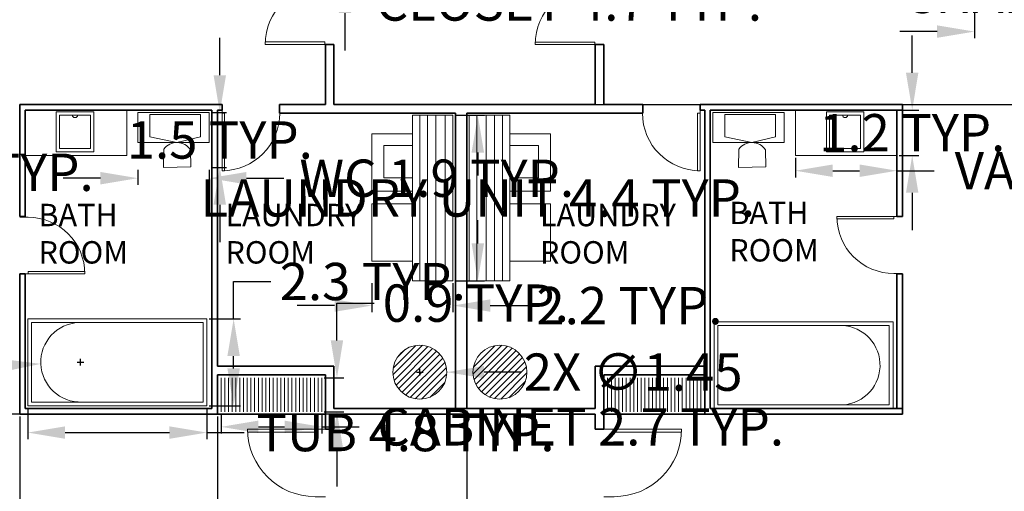
# Model space of a CAD drawing. Units: metres. Extents: x 25.1 to 96.1, y 24.3 to 71.3.
# Tile 3 of 5: x 45.8 to 72.2, y 43.8 to 56.5. Entities that reach past the tile are written whole.
import ezdxf

# ---------------------------------------------------------------- set-up
doc = ezdxf.new("R2010")
doc.units = ezdxf.units.M
doc.header["$MEASUREMENT"] = 0
for name, color, linetype, lineweight in [('A-AREA-IDEN', 1, 'Continuous', 18), ('A-EQPM', 163, 'Continuous', 18), ('A-EQPM-PATT', 152, 'Continuous', 13), ('A-FLOR-CASE', 8, 'Continuous', 18), ('A-FLOR-FIXT', 163, 'Continuous', 18), ('A-WALL', 7, 'Continuous', 35), ('dimension', 80, 'Continuous', 18), ('door', 17, 'Continuous', 18), ('furniture', 163, 'Continuous', 18)]:
    doc.layers.add(name, color=color, linetype=linetype, lineweight=lineweight)
doc.styles.get("Standard").update_dxf_attribs({"font": 'arial.ttf'})
doc.dimstyles.get("Standard").update_dxf_attribs({"dimtxt": 1, "dimasz": 1, "dimexe": 0.18, "dimexo": 0.0625, "dimgap": 0.09, "dimtad": 0, "dimtih": 1, "dimtoh": 1, "dimdec": 1, "dimzin": 0, "dimdsep": 46, "dimtxsty": 'Standard', "dimcen": 0.09, "dimadec": 0, "dimazin": 0, "dimtfac": 1, "dimtdec": 1, "dimtofl": 0, "dimtmove": 0, "dimatfit": 3, "dimfxl": 1, "dimtolj": 1, "dimtzin": 0, "dimarcsym": 0})

# ---------------------------------------------------------------- blocks, each defined once
blk = doc.blocks.new('t')
for points in [[(29.887, -1.464), (34.681, -1.464), (34.681, 0.864), (29.887, 0.864)], [(29.987, -1.364), (34.581, -1.364), (34.581, 0.764), (29.987, 0.764)]]:
    blk.add_lwpolyline(points, close=True)
blk.add_arc((31.299, -0.3), 1.065, 92.3033, 272.3033)
blk = doc.blocks.new('fff')
at = {"layer": 'furniture'}
for p, q in [((35.063, -0.715), (35.063, -1.625)), ((35.163, -0.715), (35.163, -1.625)), ((35.263, -0.715), (35.263, -1.625)), ((35.363, -0.715), (35.363, -1.625)), ((35.463, -0.715), (35.463, -1.625)), ((35.563, -0.715), (35.563, -1.625)), ((35.663, -0.715), (35.663, -1.625)), ((35.763, -0.715), (35.763, -1.625)), ((35.863, -0.715), (35.863, -1.625)), ((35.963, -0.715), (35.963, -1.625)), ((36.063, -0.715), (36.063, -1.625)), ((36.163, -0.715), (36.163, -1.625)), ((36.263, -0.715), (36.263, -1.625)), ((36.363, -0.715), (36.363, -1.625)), ((36.463, -0.715), (36.463, -1.625)), ((36.563, -0.715), (36.563, -1.625)), ((36.663, -0.715), (36.663, -1.625)), ((36.763, -0.715), (36.763, -1.625)), ((36.863, -0.715), (36.863, -1.625)), ((36.963, -0.715), (36.963, -1.625)), ((37.063, -0.715), (37.063, -1.625)), ((37.163, -0.715), (37.163, -1.625)), ((37.263, -0.715), (37.263, -1.625)), ((37.363, -0.715), (37.363, -1.625)), ((37.463, -0.715), (37.463, -1.625)), ((37.563, -0.715), (37.563, -1.625)), ((37.663, -0.715), (37.663, -1.625)), ((37.763, -0.715), (37.763, -1.625))]:
    blk.add_line(p, q, dxfattribs=at)
blk = doc.blocks.new('sinn')
for points in [[(29.82, 6.458), (32.54, 6.458), (32.54, 5.24), (29.82, 5.24)], [(30.649, 6.409), (31.653, 6.409), (31.653, 5.34), (30.649, 5.34)], [(30.734, 6.324), (31.567, 6.324), (31.567, 5.426), (30.734, 5.426)]]:
    blk.add_lwpolyline(points, close=True)
blk.add_arc((31.151, 6.324), 0.0703, 180, 0)
blk = doc.blocks.new('wc')
for p, q in [((33.157, 5.739), (33.883, 5.588)), ((33.883, 5.588), (34.514, 5.739)), ((33.535, 5.411), (33.522, 4.918)), ((34.255, 4.935), (34.244, 5.394)), ((33.522, 4.918), (34.255, 4.935))]:
    blk.add_line(p, q)
blk.add_lwpolyline([(32.833, 6.392), (34.743, 6.392), (34.743, 5.588), (32.833, 5.588)], close=True)
blk.add_lwpolyline([(33.157, 5.739), (33.157, 6.335), (34.514, 6.335), (34.514, 5.739)])
blk.add_arc((33.883, 5.156), 0.432, 33.4958, 143.723)
blk = doc.blocks.new('w')
at = {"layer": 'furniture'}
for p, q in [((40.384, 1.885), (40.384, 6.319)), ((40.596, 1.885), (40.596, 6.319)), ((40.82, 1.885), (40.82, 6.319)), ((40.82, 1.885), (40.82, 6.319)), ((41.069, 1.885), (41.069, 6.319))]:
    blk.add_line(p, q, dxfattribs=at)
for points in [[(41.275, 6.319), (40.188, 6.319), (40.188, 1.885), (41.275, 1.885)], [(40.188, 5.819), (39.103, 5.819), (39.103, 4.287), (40.188, 4.287)], [(40.188, 5.51), (39.421, 5.51), (39.421, 4.637), (40.188, 4.637)], [(40.188, 3.945), (39.103, 3.945), (39.103, 2.413), (40.188, 2.413)]]:
    blk.add_lwpolyline(points, close=True, dxfattribs=at)
blk = doc.blocks.new('*U22')
for p, q in [((0, 0), (0, -6)), ((40, 0), (40, -6))]:
    blk.add_line(p, q)
blk.add_lwpolyline([(0, 0), (0, 40), (1.75, 40), (1.75, 0)], close=True)
blk.add_arc((0, 0), 40, 0, 90)
blk = doc.blocks.new('*D34')
at = {"layer": 'Defpoints', "color": 0, "transparency": 16777216}
for p in [(46.002, 46.126), (50.795, 46.126), (50.795, 45.407)]:
    blk.add_point(p, dxfattribs=at)
at = {"layer": 'dimension', "color": 0, "lineweight": -2, "transparency": 16777216}
for p, q in [((46.002, 46.063), (46.002, 45.227)), ((50.795, 46.063), (50.795, 45.227)), ((47.002, 45.407), (49.795, 45.407)), ((50.795, 45.407), (51.795, 45.407))]:
    blk.add_line(p, q, dxfattribs=at)
at = {"layer": 'dimension', "color": 0, "transparency": 16777216}
for points in [[(47.002, 45.573), (47.002, 45.24), (46.002, 45.407)], [(49.795, 45.573), (49.795, 45.24), (50.795, 45.407)]]:
    blk.add_solid(points, dxfattribs=at)
at = {"layer": 'dimension', "color": 0, "transparency": 16777216, "insert": (56.117, 45.407), "char_height": 1, "attachment_point": 5}
blk.add_mtext('\\A1;TUB 4.8 TYP.', dxfattribs=at)
blk = doc.blocks.new('*D35')
at = {"layer": 'Defpoints', "color": 0, "transparency": 16777216}
for p in [(50.795, 48.454), (51.514, 48.454), (50.795, 46.126)]:
    blk.add_point(p, dxfattribs=at)
at = {"layer": 'dimension', "color": 0, "lineweight": -2, "transparency": 16777216}
for p, q in [((51.514, 48.454), (51.514, 49.454)), ((51.514, 49.454), (52.514, 49.454)), ((50.858, 48.454), (51.694, 48.454)), ((51.514, 47.126), (51.514, 47.454)), ((50.858, 46.126), (51.694, 46.126))]:
    blk.add_line(p, q, dxfattribs=at)
at = {"layer": 'dimension', "color": 0, "transparency": 16777216}
for points in [[(51.347, 47.454), (51.681, 47.454), (51.514, 48.454)], [(51.347, 47.126), (51.681, 47.126), (51.514, 46.126)]]:
    blk.add_solid(points, dxfattribs=at)
at = {"layer": 'dimension', "color": 0, "transparency": 16777216, "insert": (55.24, 49.454), "char_height": 1, "attachment_point": 5}
blk.add_mtext('\\A1;2.3 TYP.', dxfattribs=at)
blk = doc.blocks.new('*D37')
at = {"layer": 'Defpoints', "color": 0, "transparency": 16777216}
for p in [(71.357, 57.619), (72.431, 57.619), (72.431, 56.149)]:
    blk.add_point(p, dxfattribs=at)
at = {"layer": 'dimension', "color": 0, "lineweight": -2, "transparency": 16777216}
for p, q in [((71.357, 57.557), (71.357, 55.969)), ((72.431, 57.557), (72.431, 55.969)), ((70.357, 56.149), (69.357, 56.149)), ((73.431, 56.149), (74.431, 56.149))]:
    blk.add_line(p, q, dxfattribs=at)
at = {"layer": 'dimension', "color": 0, "transparency": 16777216}
for points in [[(70.357, 56.316), (70.357, 55.982), (71.357, 56.149)], [(73.431, 56.316), (73.431, 55.982), (72.431, 56.149)]]:
    blk.add_solid(points, dxfattribs=at)
at = {"layer": 'dimension', "color": 0, "transparency": 16777216, "insert": (77.102, 56.149), "char_height": 1, "attachment_point": 5}
blk.add_mtext('\\A1;1.1 TYP.', dxfattribs=at)
blk = doc.blocks.new('*D44')
at = {"layer": 'Defpoints', "color": 0, "transparency": 16777216}
for p in [(35.843, 52.744), (38.271, 52.744), (38.271, 52.38)]:
    blk.add_point(p, dxfattribs=at)
at = {"layer": 'dimension', "color": 0, "lineweight": -2, "transparency": 16777216}
for p, q in [((35.843, 52.682), (35.843, 52.2)), ((38.271, 52.682), (38.271, 52.2)), ((36.843, 52.38), (37.271, 52.38)), ((38.271, 52.38), (39.271, 52.38))]:
    blk.add_line(p, q, dxfattribs=at)
at = {"layer": 'dimension', "color": 0, "transparency": 16777216}
for points in [[(36.843, 52.547), (36.843, 52.213), (35.843, 52.38)], [(37.271, 52.547), (37.271, 52.213), (38.271, 52.38)]]:
    blk.add_solid(points, dxfattribs=at)
at = {"layer": 'dimension', "color": 0, "transparency": 16777216, "insert": (43.67, 52.38), "char_height": 1, "attachment_point": 5}
blk.add_mtext('\\A1;HOB 2.4 TYP.', dxfattribs=at)
blk = doc.blocks.new('*D48')
at = {"layer": 'Defpoints', "color": 0, "transparency": 16777216}
for p in [(80.148, 57.146), (80.148, 56.81), (82.383, 56.81)]:
    blk.add_point(p, dxfattribs=at)
at = {"layer": 'dimension', "color": 0, "lineweight": -2, "transparency": 16777216}
for p, q in [((80.148, 56.873), (80.148, 57.326)), ((82.383, 56.873), (82.383, 57.326)), ((80.148, 57.146), (79.148, 57.146)), ((81.383, 57.146), (81.148, 57.146))]:
    blk.add_line(p, q, dxfattribs=at)
at = {"layer": 'dimension', "color": 0, "transparency": 16777216}
for points in [[(81.148, 57.312), (81.148, 56.979), (80.148, 57.146)], [(81.383, 57.312), (81.383, 56.979), (82.383, 57.146)]]:
    blk.add_solid(points, dxfattribs=at)
at = {"layer": 'dimension', "color": 0, "transparency": 16777216, "insert": (74.068, 57.146), "char_height": 1, "attachment_point": 5}
blk.add_mtext('\\A1;CHAIR 2.2 TYP.', dxfattribs=at)
blk = doc.blocks.new('*D56')
at = {"layer": 'Defpoints', "color": 0, "transparency": 16777216}
for p in [(49.092, 57.646), (53.792, 57.646), (53.792, 56.941)]:
    blk.add_point(p, dxfattribs=at)
at = {"layer": 'dimension', "color": 0, "lineweight": -2, "transparency": 16777216}
for p, q in [((49.092, 57.584), (49.092, 56.761)), ((53.792, 57.584), (53.792, 56.761)), ((50.092, 56.941), (52.792, 56.941)), ((53.792, 56.941), (54.792, 56.941))]:
    blk.add_line(p, q, dxfattribs=at)
at = {"layer": 'dimension', "color": 0, "transparency": 16777216}
for points in [[(50.092, 57.108), (50.092, 56.774), (49.092, 56.941)], [(52.792, 57.108), (52.792, 56.774), (53.792, 56.941)]]:
    blk.add_solid(points, dxfattribs=at)
at = {"layer": 'dimension', "color": 0, "transparency": 16777216, "insert": (60.493, 56.941), "char_height": 1, "attachment_point": 5}
blk.add_mtext('\\A1;CLOSET 4.7 TYP.', dxfattribs=at)
blk = doc.blocks.new('*D57')
at = {"layer": 'Defpoints', "color": 0, "transparency": 16777216}
for p in [(53.792, 58.716), (54.497, 58.716), (53.792, 57.646)]:
    blk.add_point(p, dxfattribs=at)
at = {"layer": 'dimension', "color": 0, "lineweight": -2, "transparency": 16777216}
for p, q in [((54.497, 59.716), (54.497, 60.716)), ((54.497, 60.716), (55.497, 60.716)), ((53.855, 58.716), (54.677, 58.716)), ((53.855, 57.646), (54.677, 57.646)), ((54.497, 56.646), (54.497, 55.646))]:
    blk.add_line(p, q, dxfattribs=at)
at = {"layer": 'dimension', "color": 0, "transparency": 16777216}
for points in [[(54.331, 59.716), (54.664, 59.716), (54.497, 58.716)], [(54.331, 56.646), (54.664, 56.646), (54.497, 57.646)]]:
    blk.add_solid(points, dxfattribs=at)
at = {"layer": 'dimension', "color": 0, "transparency": 16777216, "insert": (58.168, 60.716), "char_height": 1, "attachment_point": 5}
blk.add_mtext('\\A1;1.1 TYP.', dxfattribs=at)
blk = doc.blocks.new('*D58')
at = {"layer": 'Defpoints', "color": 0, "transparency": 16777216}
for p in [(51.177, 45.965), (53.877, 45.965), (53.877, 45.56)]:
    blk.add_point(p, dxfattribs=at)
at = {"layer": 'dimension', "color": 0, "lineweight": -2, "transparency": 16777216}
for p, q in [((51.177, 45.903), (51.177, 45.38)), ((53.877, 45.903), (53.877, 45.38)), ((52.177, 45.56), (52.877, 45.56)), ((53.877, 45.56), (54.877, 45.56))]:
    blk.add_line(p, q, dxfattribs=at)
at = {"layer": 'dimension', "color": 0, "transparency": 16777216}
for points in [[(52.177, 45.727), (52.177, 45.394), (51.177, 45.56)], [(52.877, 45.727), (52.877, 45.394), (53.877, 45.56)]]:
    blk.add_solid(points, dxfattribs=at)
at = {"layer": 'dimension', "color": 0, "transparency": 16777216, "insert": (60.81, 45.56), "char_height": 1, "attachment_point": 5}
blk.add_mtext('\\A1;CABINET 2.7 TYP.', dxfattribs=at)
blk = doc.blocks.new('*D59')
at = {"layer": 'Defpoints', "color": 0, "transparency": 16777216}
for p in [(53.877, 46.875), (54.282, 46.875), (53.877, 45.965)]:
    blk.add_point(p, dxfattribs=at)
at = {"layer": 'dimension', "color": 0, "lineweight": -2, "transparency": 16777216}
for p, q in [((54.282, 47.875), (54.282, 48.875)), ((54.282, 48.875), (55.282, 48.875)), ((53.939, 46.875), (54.462, 46.875)), ((53.939, 45.965), (54.462, 45.965)), ((54.282, 44.965), (54.282, 43.965))]:
    blk.add_line(p, q, dxfattribs=at)
at = {"layer": 'dimension', "color": 0, "transparency": 16777216}
for points in [[(54.115, 47.875), (54.448, 47.875), (54.282, 46.875)], [(54.115, 44.965), (54.448, 44.965), (54.282, 45.965)]]:
    blk.add_solid(points, dxfattribs=at)
at = {"layer": 'dimension', "color": 0, "transparency": 16777216, "insert": (58, 48.875), "char_height": 1, "attachment_point": 5}
blk.add_mtext('\\A1;0.9 TYP.', dxfattribs=at)
blk = doc.blocks.new('*D60')
at = {"layer": 'Defpoints', "color": 0, "transparency": 16777216}
for p in [(66.561, 52.83), (69.281, 52.83), (69.281, 52.422)]:
    blk.add_point(p, dxfattribs=at)
at = {"layer": 'dimension', "color": 0, "lineweight": -2, "transparency": 16777216}
for p, q in [((66.561, 52.767), (66.561, 52.242)), ((69.281, 52.767), (69.281, 52.242)), ((67.561, 52.422), (68.281, 52.422)), ((69.281, 52.422), (70.281, 52.422))]:
    blk.add_line(p, q, dxfattribs=at)
at = {"layer": 'dimension', "color": 0, "transparency": 16777216}
for points in [[(67.561, 52.588), (67.561, 52.255), (66.561, 52.422)], [(68.281, 52.588), (68.281, 52.255), (69.281, 52.422)]]:
    blk.add_solid(points, dxfattribs=at)
at = {"layer": 'dimension', "color": 0, "transparency": 16777216, "insert": (75.742, 52.422), "char_height": 1, "attachment_point": 5}
blk.add_mtext('\\A1;VANITY 2.7 TYP.', dxfattribs=at)
blk = doc.blocks.new('*D61')
at = {"layer": 'Defpoints', "color": 0, "transparency": 16777216}
for p in [(69.281, 54.048), (69.689, 54.048), (69.281, 52.83)]:
    blk.add_point(p, dxfattribs=at)
at = {"layer": 'dimension', "color": 0, "lineweight": -2, "transparency": 16777216}
for p, q in [((69.689, 55.048), (69.689, 56.048)), ((69.343, 54.048), (69.869, 54.048)), ((69.343, 52.83), (69.869, 52.83)), ((69.689, 51.83), (69.689, 50.83))]:
    blk.add_line(p, q, dxfattribs=at)
at = {"layer": 'dimension', "color": 0, "transparency": 16777216}
for points in [[(69.522, 55.048), (69.855, 55.048), (69.689, 54.048)], [(69.522, 51.83), (69.855, 51.83), (69.689, 52.83)]]:
    blk.add_solid(points, dxfattribs=at)
at = {"layer": 'dimension', "color": 0, "transparency": 16777216, "insert": (69.689, 53.439), "char_height": 1, "attachment_point": 5}
blk.add_mtext('\\A1;1.2 TYP.', dxfattribs=at)
blk = doc.blocks.new('*D62')
at = {"layer": 'Defpoints', "color": 0, "transparency": 16777216}
for p in [(48.947, 52.508), (50.857, 52.508), (50.857, 52.221)]:
    blk.add_point(p, dxfattribs=at)
at = {"layer": 'dimension', "color": 0, "lineweight": -2, "transparency": 16777216}
for p, q in [((47.947, 52.221), (46.947, 52.221)), ((48.947, 52.446), (48.947, 52.041)), ((50.857, 52.446), (50.857, 52.041)), ((51.857, 52.221), (52.857, 52.221))]:
    blk.add_line(p, q, dxfattribs=at)
at = {"layer": 'dimension', "color": 0, "transparency": 16777216}
for points in [[(47.947, 52.388), (47.947, 52.055), (48.947, 52.221)], [(51.857, 52.388), (51.857, 52.055), (50.857, 52.221)]]:
    blk.add_solid(points, dxfattribs=at)
at = {"layer": 'dimension', "color": 0, "transparency": 16777216, "insert": (56.954, 52.221), "char_height": 1, "attachment_point": 5}
blk.add_mtext('\\A1;WC 1.9 TYP.', dxfattribs=at)
blk = doc.blocks.new('*D63')
at = {"layer": 'Defpoints', "color": 0, "transparency": 16777216}
for p in [(50.857, 53.981), (51.144, 53.981), (50.857, 52.508)]:
    blk.add_point(p, dxfattribs=at)
at = {"layer": 'dimension', "color": 0, "lineweight": -2, "transparency": 16777216}
for p, q in [((51.144, 54.981), (51.144, 55.981)), ((50.92, 53.981), (51.324, 53.981)), ((50.92, 52.508), (51.324, 52.508)), ((51.144, 51.508), (51.144, 50.508))]:
    blk.add_line(p, q, dxfattribs=at)
at = {"layer": 'dimension', "color": 0, "transparency": 16777216}
for points in [[(50.977, 54.981), (51.311, 54.981), (51.144, 53.981)], [(50.977, 51.508), (51.311, 51.508), (51.144, 52.508)]]:
    blk.add_solid(points, dxfattribs=at)
at = {"layer": 'dimension', "color": 0, "transparency": 16777216, "insert": (51.144, 53.245), "char_height": 1, "attachment_point": 5}
blk.add_mtext('\\A1;1.5 TYP.', dxfattribs=at)
blk = doc.blocks.new('*D64')
at = {"layer": 'Defpoints', "color": 0, "transparency": 16777216}
for p in [(57.389, 53.909), (58.055, 53.909), (57.389, 49.475)]:
    blk.add_point(p, dxfattribs=at)
at = {"layer": 'dimension', "color": 0, "lineweight": -2, "transparency": 16777216}
for p, q in [((57.452, 53.909), (58.235, 53.909)), ((58.055, 52.909), (58.055, 52.29)), ((58.055, 50.475), (58.055, 51.093)), ((57.452, 49.475), (58.235, 49.475))]:
    blk.add_line(p, q, dxfattribs=at)
at = {"layer": 'dimension', "color": 0, "transparency": 16777216}
for points in [[(57.888, 52.909), (58.221, 52.909), (58.055, 53.909)], [(57.888, 50.475), (58.221, 50.475), (58.055, 49.475)]]:
    blk.add_solid(points, dxfattribs=at)
at = {"layer": 'dimension', "color": 0, "transparency": 16777216, "insert": (58.055, 51.692), "char_height": 1, "attachment_point": 5}
blk.add_mtext('\\A1;LAUNDRY UNIT 4.4 TYP.', dxfattribs=at)
blk = doc.blocks.new('*D65')
at = {"layer": 'Defpoints', "color": 0, "transparency": 16777216}
for p in [(55.217, 49.475), (57.389, 49.475), (57.389, 48.809)]:
    blk.add_point(p, dxfattribs=at)
at = {"layer": 'dimension', "color": 0, "lineweight": -2, "transparency": 16777216}
for p, q in [((55.217, 49.412), (55.217, 48.629)), ((57.389, 49.412), (57.389, 48.629)), ((54.217, 48.809), (53.217, 48.809)), ((58.389, 48.809), (59.389, 48.809))]:
    blk.add_line(p, q, dxfattribs=at)
at = {"layer": 'dimension', "color": 0, "transparency": 16777216}
for points in [[(54.217, 48.976), (54.217, 48.643), (55.217, 48.809)], [(58.389, 48.976), (58.389, 48.643), (57.389, 48.809)]]:
    blk.add_solid(points, dxfattribs=at)
at = {"layer": 'dimension', "color": 0, "transparency": 16777216, "insert": (62.116, 48.809), "char_height": 1, "attachment_point": 5}
blk.add_mtext('\\A1;2.2 TYP.', dxfattribs=at)
blk = doc.blocks.new('*D78')
at = {"layer": 'Defpoints', "color": 0, "transparency": 16777216}
for p in [(45.784, 45.898), (51.084, 45.898), (51.084, 24.973)]:
    blk.add_point(p, dxfattribs=at)
at = {"layer": 'dimension', "color": 0, "lineweight": -2, "transparency": 16777216}
for p, q in [((45.784, 45.835), (45.784, 24.793)), ((51.084, 45.835), (51.084, 24.793)), ((46.784, 24.973), (47.434, 24.973)), ((50.084, 24.973), (49.434, 24.973))]:
    blk.add_line(p, q, dxfattribs=at)
at = {"layer": 'dimension', "color": 0, "transparency": 16777216}
for points in [[(46.784, 25.139), (46.784, 24.806), (45.784, 24.973)], [(50.084, 25.139), (50.084, 24.806), (51.084, 24.973)]]:
    blk.add_solid(points, dxfattribs=at)
at = {"layer": 'dimension', "color": 0, "transparency": 16777216, "insert": (48.434, 24.973), "char_height": 1, "attachment_point": 5}
blk.add_mtext('\\A1;5.3', dxfattribs=at)
blk = doc.blocks.new('*D79')
at = {"layer": 'Defpoints', "color": 0, "transparency": 16777216}
for p in [(51.084, 45.898), (57.757, 46.048), (57.757, 24.973)]:
    blk.add_point(p, dxfattribs=at)
at = {"layer": 'dimension', "color": 0, "lineweight": -2, "transparency": 16777216}
for p, q in [((57.757, 45.985), (57.757, 24.793)), ((51.084, 45.835), (51.084, 24.793)), ((52.084, 24.973), (52.641, 24.973)), ((56.757, 24.973), (56.201, 24.973))]:
    blk.add_line(p, q, dxfattribs=at)
at = {"layer": 'dimension', "color": 0, "transparency": 16777216}
for points in [[(52.084, 25.139), (52.084, 24.806), (51.084, 24.973)], [(56.757, 25.139), (56.757, 24.806), (57.757, 24.973)]]:
    blk.add_solid(points, dxfattribs=at)
at = {"layer": 'dimension', "color": 0, "transparency": 16777216, "insert": (54.421, 24.973), "char_height": 1, "attachment_point": 5}
blk.add_mtext('\\A1;6.673', dxfattribs=at)
blk = doc.blocks.new('*D84')
at = {"layer": 'Defpoints', "color": 0, "transparency": 16777216}
for p in [(29.225, 45.898), (61.201, 45.898), (61.201, 32.464)]:
    blk.add_point(p, dxfattribs=at)
at = {"layer": 'dimension', "color": 0, "lineweight": -2, "transparency": 16777216}
for p, q in [((61.138, 45.898), (29.045, 45.898)), ((29.225, 44.898), (29.225, 39.781)), ((29.225, 33.464), (29.225, 38.58)), ((61.138, 32.464), (29.045, 32.464))]:
    blk.add_line(p, q, dxfattribs=at)
at = {"layer": 'dimension', "color": 0, "transparency": 16777216}
for points in [[(29.059, 44.898), (29.392, 44.898), (29.225, 45.898)], [(29.059, 33.464), (29.392, 33.464), (29.225, 32.464)]]:
    blk.add_solid(points, dxfattribs=at)
at = {"layer": 'dimension', "color": 0, "transparency": 16777216, "insert": (29.225, 39.181), "char_height": 1, "attachment_point": 5}
blk.add_mtext('\\A1;13.434', dxfattribs=at)
blk = doc.blocks.new('*D85')
at = {"layer": 'Defpoints', "color": 0, "transparency": 16777216}
for p in [(54.201, 67.782), (86.176, 67.782), (54.201, 54.198)]:
    blk.add_point(p, dxfattribs=at)
at = {"layer": 'dimension', "color": 0, "lineweight": -2, "transparency": 16777216}
for p, q in [((54.263, 67.782), (86.356, 67.782)), ((86.176, 66.782), (86.176, 61.59)), ((86.176, 55.198), (86.176, 60.389)), ((54.263, 54.198), (86.356, 54.198))]:
    blk.add_line(p, q, dxfattribs=at)
at = {"layer": 'dimension', "color": 0, "transparency": 16777216}
for points in [[(86.009, 66.782), (86.342, 66.782), (86.176, 67.782)], [(86.009, 55.198), (86.342, 55.198), (86.176, 54.198)]]:
    blk.add_solid(points, dxfattribs=at)
at = {"layer": 'dimension', "color": 0, "transparency": 16777216, "insert": (86.176, 60.99), "char_height": 1, "attachment_point": 5}
blk.add_mtext('\\A1;13.584', dxfattribs=at)
blk = doc.blocks.new('*D87')
at = {"layer": 'Defpoints', "color": 0, "transparency": 16777216}
for p in [(55.777, 47.024), (57.224, 47.025)]:
    blk.add_point(p, dxfattribs=at)
at = {"layer": 'dimension', "color": 0, "lineweight": -2, "transparency": 16777216}
for p, q in [((56.411, 47.025), (56.591, 47.025)), ((56.501, 46.935), (56.501, 47.115)), ((59.224, 47.026), (58.224, 47.025))]:
    blk.add_line(p, q, dxfattribs=at)
at = {"layer": 'dimension', "color": 0, "transparency": 16777216}
blk.add_solid([(58.224, 47.192), (58.224, 46.859), (57.224, 47.025)], dxfattribs=at)
at = {"layer": 'dimension', "color": 0, "transparency": 16777216, "insert": (62.216, 47.026), "char_height": 1, "attachment_point": 5}
blk.add_mtext('\\A1;2X ∅1.45', dxfattribs=at)
blk = doc.blocks.new('*D88')
at = {"layer": 'Defpoints', "color": 0, "transparency": 16777216}
for p in [(46.349, 47.247), (47.413, 47.29)]:
    blk.add_point(p, dxfattribs=at)
at = {"layer": 'dimension', "color": 0, "lineweight": -2, "transparency": 16777216}
for p, q in [((44.351, 47.166), (45.35, 47.207)), ((47.323, 47.29), (47.503, 47.29)), ((47.413, 47.2), (47.413, 47.38))]:
    blk.add_line(p, q, dxfattribs=at)
at = {"layer": 'dimension', "color": 0, "transparency": 16777216}
blk.add_solid([(45.344, 47.373), (45.357, 47.04), (46.349, 47.247)], dxfattribs=at)
at = {"layer": 'dimension', "color": 0, "transparency": 16777216, "insert": (41.009, 47.166), "char_height": 1, "attachment_point": 5}
blk.add_mtext('\\A1;2X R1.065', dxfattribs=at)

msp = doc.modelspace()

# ---------------------------------------------------------------- hatches: boundary and pattern name
at = {"layer": 'A-EQPM-PATT'}
h = msp.add_hatch(dxfattribs=at)
h.set_pattern_fill('ANSI31', color=256)
h.set_pattern_definition([(45, (16.1141, 47.58982), (-0.08838835, 0.08838835), [])])
h.paths.add_polyline_path([(57.2236, 47.0247, 1), (55.7774, 47.0247, 1)])
h.paths.add_polyline_path([(59.3692, 47.0247, 1), (57.923, 47.0247, 1)])

# ---------------------------------------------------------------- linework, layer by layer
at = {"layer": 'A-EQPM'}
for centre in [(56.5005, 47.0247), (58.6461, 47.0247)]:
    msp.add_circle(centre, 0.7231, dxfattribs=at)
at = {"layer": 'A-WALL'}
for p, q in [((53.9708, 55.8), (54.2008, 55.8)), ((61.2008, 55.8), (61.4308, 55.8)), ((45.7841, 54.1975), (51.2035, 54.1975)), ((45.7841, 54.1975), (45.7841, 51.3532)), ((51.2035, 54.0475), (51.2035, 54.1975)), ((52.7435, 54.1975), (53.9708, 54.1975)), ((52.7435, 53.9675), (52.7435, 54.1975)), ((54.2008, 54.1975), (61.2008, 54.1975)), ((61.4308, 54.1975), (62.4701, 54.1975)), ((62.4701, 53.9675), (62.4701, 54.1975)), ((64.0101, 54.0475), (64.0101, 54.1975)), ((64.0101, 54.1975), (69.4308, 54.1975)), ((69.4308, 54.1975), (69.4308, 51.196)), ((45.9341, 54.0475), (50.9341, 54.0475)), ((45.9341, 54.0475), (45.9341, 51.3532)), ((50.9341, 54.0475), (50.9341, 46.0475)), ((51.0841, 54.0475), (51.0841, 47.1875)), ((51.0841, 54.0475), (51.2035, 54.0475)), ((52.7435, 53.9675), (57.4574, 53.9675)), ((57.4574, 46.0475), (57.4574, 53.9675)), ((57.7574, 46.0475), (57.7574, 53.9675)), ((57.7574, 53.9675), (62.4701, 53.9675)), ((64.0101, 54.0475), (64.1308, 54.0475)), ((64.1308, 54.0475), (64.1308, 47.1875)), ((64.2808, 54.0475), (64.2808, 46.0475)), ((64.2808, 54.0475), (69.4308, 54.0475)), ((69.2808, 54.0475), (69.2808, 51.196)), ((45.7841, 51.3532), (45.7841, 51.196)), ((45.9341, 51.196), (45.7841, 51.196)), ((45.9341, 51.3532), (45.9341, 51.196)), ((69.2808, 51.196), (69.4308, 51.196)), ((45.7841, 49.656), (45.7841, 45.8975)), ((45.9341, 49.656), (45.7841, 49.656)), ((45.9341, 49.656), (45.9341, 46.0475)), ((69.2808, 49.656), (69.2808, 46.0475)), ((69.2808, 49.656), (69.4308, 49.656)), ((69.4308, 49.656), (69.4308, 45.8975)), ((54.2008, 47.1875), (51.0841, 47.1875)), ((53.9708, 46.9575), (51.0841, 46.9575)), ((51.0841, 46.9575), (51.0841, 46.0475)), ((53.9708, 46.9575), (53.9708, 45.5013)), ((54.2008, 47.1875), (54.2008, 46.0475)), ((61.2008, 47.1875), (61.2008, 46.0475)), ((64.1308, 47.1875), (61.2008, 47.1875)), ((61.4308, 46.9575), (61.4308, 46.0475)), ((64.1308, 46.9575), (61.4308, 46.9575)), ((64.1308, 46.9575), (64.1308, 46.0475)), ((51.0841, 45.8975), (45.7841, 45.8975)), ((50.9341, 46.0475), (45.9341, 46.0475)), ((51.0841, 46.0475), (51.0841, 45.8975)), ((51.0841, 45.8975), (53.9708, 45.8975)), ((61.2008, 46.0475), (54.2008, 46.0475)), ((61.2008, 45.8975), (54.2008, 45.8975)), ((54.2008, 45.8975), (54.2008, 45.5013)), ((61.2008, 45.8975), (61.2008, 45.5013)), ((61.4308, 46.0475), (61.4308, 45.8975)), ((61.4308, 45.8975), (61.4308, 45.5013)), ((64.1308, 45.8975), (61.4308, 45.8975)), ((64.1308, 46.0475), (64.1308, 45.8975)), ((69.4308, 45.8975), (64.1308, 45.8975)), ((69.4308, 46.0475), (64.2808, 46.0475)), ((53.9708, 45.5013), (54.2008, 45.5013)), ((61.2008, 45.5013), (61.4308, 45.5013))]:
    msp.add_line(p, q, dxfattribs=at)
for points in [[(53.9708, 55.8), (53.9708, 54.1975)], [(54.2008, 54.1975), (54.2008, 55.8)], [(61.2008, 55.8), (61.2008, 54.1975)], [(61.4308, 54.1975), (61.4308, 55.8)]]:
    msp.add_lwpolyline(points, dxfattribs=at)

# ---------------------------------------------------------------- block references
at = {"layer": 'A-EQPM'}
msp.add_blockref('w', (16.1141, 47.5898), dxfattribs=at)
at = {"layer": 'A-EQPM', "xscale": -1}
msp.add_blockref('w', (99.1008, 47.5898), dxfattribs=at)
at = {"layer": 'A-FLOR-CASE'}
for p in [(16.1141, 47.5898), (26.3682, 47.5898)]:
    msp.add_blockref('fff', p, dxfattribs=at)
at = {"layer": 'A-FLOR-FIXT'}
for name, p in [('sinn', (16.1141, 47.5898)), ('wc', (16.1141, 47.5898)), ('wc', (31.514, 47.5898)), ('sinn', (36.7411, 47.5898)), ('t', (16.1141, 47.5898)), ('t', (16.1141, 47.5898))]:
    msp.add_blockref(name, p, dxfattribs=at)
at = {"layer": 'A-FLOR-FIXT', "xscale": -1}
msp.add_blockref('t', (99.0618, 47.5115), dxfattribs=at)
at = {"layer": 'door'}
for p, xscale, yscale, zscale, rotation in [((53.9604, 55.8), 0.0400617254265443, 0.0400617254265443, 0.0400617254265443, 90), ((61.1909, 55.8), 0.0399749143269108, 0.0399749143269108, 0.0399749143269108, 90), ((51.2035, 53.9657), -0.0386448922260039, 0.0386448922260039, 0.0386448922260039, 180), ((64.0101, 53.9657), 0.0386448922260039, 0.0386448922260039, 0.0386448922260039, 180), ((46.0118, 49.656), -0.0379497194996768, 0.0379497194996768, 0.0379497194996768, 269.9999999999993), ((69.2014, 51.196), -0.0382357842374183, 0.0382357842374183, 0.0382357842374183, 90), ((53.6991, 45.5013), -0.0452901221034344, 0.0452901221034344, 0.0452901221034344, 90), ((61.7025, 45.5013), 0.0452901221034344, 0.0452901221034344, 0.0452901221034344, 270)]:
    msp.add_blockref('*U22', p, dxfattribs=dict(at, xscale=xscale, yscale=yscale, zscale=zscale, rotation=rotation))

# ---------------------------------------------------------------- texts
at = {"layer": 'A-AREA-IDEN', "char_height": 0.6, "attachment_point": 1}
for s, insert in [('BATH\\PROOM', (46.2877, 51.535)), ('LAUNDRY\\PROOM', (51.2949, 51.535)), ('LAUNDRY\\PROOM', (59.719, 51.535)), ('BATH\\PROOM', (64.7895, 51.59))]:
    msp.add_mtext_dynamic_manual_height_columns(s, width=5.007262, gutter_width=1, heights=[0], dxfattribs=dict(at, insert=insert))

# ---------------------------------------------------------------- dimensions: what is measured, and where the dimension line sits
at = {"layer": 'dimension'}
for base, p1, p2, picture, middle in [((86.1758, 67.7816), (54.2008, 54.1975), (54.2008, 67.7816), '*D85', (86.1758, 60.9895)), ((29.2252, 45.8975), (61.2008, 32.4635), (61.2008, 45.8975), '*D84', (29.2252, 39.1805))]:
    dim = msp.add_linear_dim(base=base, p1=p1, p2=p2, angle=90, dimstyle='Standard', override={"dimdec": 3, "dimlfac": 1, "dimrnd": 0, "dimzin": 0, "dimdsep": 46, "dimlunit": 2}, dxfattribs=at)
    dim.commit()
    dim.dimension.update_dxf_attribs({"geometry": picture, "text_midpoint": middle})
for base, p1, p2, angle, text, picture, middle in [((54.4975, 58.7156), (53.7925, 57.6461), (53.7925, 58.7156), 90, '<> TYP.', '*D57', (58.1683, 60.7156)), ((80.1479, 57.1455), (82.383, 56.8102), (80.1479, 56.8102), 180, 'CHAIR <> TYP.', '*D48', (74.0685, 57.1455)), ((51.1441, 53.9814), (50.8575, 52.508), (50.8575, 53.9814), 90, '<> TYP.', '*D63', (51.1441, 53.2447)), ((69.6887, 54.0475), (69.2808, 52.8295), (69.2808, 54.0475), 90, '<> TYP.', '*D61', (69.6887, 53.4385)), ((58.0546, 53.9092), (57.3894, 49.4745), (57.3894, 53.9092), 90, 'LAUNDRY UNIT <> TYP.', '*D64', (58.0546, 51.6919)), ((51.514, 48.454), (50.795, 46.1258), (50.795, 48.454), 90, '<> TYP.', '*D35', (55.2405, 49.454)), ((54.2816, 46.8747), (53.8766, 45.9652), (53.8766, 46.8747), 90, '<> TYP.', '*D59', (57.9995, 48.8747))]:
    dim = msp.add_linear_dim(base=base, p1=p1, p2=p2, angle=angle, text=text, dimstyle='Standard', override={"dimdec": 1, "dimlfac": 1, "dimrnd": 0, "dimzin": 0, "dimdsep": 46, "dimlunit": 2}, dxfattribs=at)
    dim.commit()
    dim.dimension.update_dxf_attribs({"geometry": picture, "text_midpoint": middle})
for base, p1, p2, text, picture, middle in [((53.7925, 56.9411), (49.0925, 57.6461), (53.7925, 57.6461), 'CLOSET <> TYP.', '*D56', (60.4933, 56.9411)), ((72.4312, 56.1491), (71.3574, 57.6191), (72.4312, 57.6191), '<> TYP.', '*D37', (77.1021, 56.1491)), ((38.2712, 52.3801), (35.8431, 52.7443), (38.2712, 52.7443), 'HOB <> TYP.', '*D44', (43.6698, 52.3801)), ((69.2808, 52.4216), (66.5611, 52.8295), (69.2808, 52.8295), 'VANITY <> TYP.', '*D60', (75.7415, 52.4216)), ((50.8575, 52.2214), (48.9467, 52.508), (50.8575, 52.508), 'WC <> TYP.', '*D62', (56.9536, 52.2214)), ((57.3894, 48.8093), (55.217, 49.4745), (57.3894, 49.4745), '<> TYP.', '*D65', (62.1158, 48.8093)), ((50.795, 45.4068), (46.0015, 46.1258), (50.795, 46.1258), 'TUB <> TYP.', '*D34', (56.1166, 45.4068)), ((53.8766, 45.5602), (51.1766, 45.9652), (53.8766, 45.9652), 'CABINET <> TYP.', '*D58', (60.8101, 45.5602))]:
    dim = msp.add_linear_dim(base=base, p1=p1, p2=p2, text=text, dimstyle='Standard', override={"dimdec": 1, "dimlfac": 1, "dimrnd": 0, "dimzin": 0, "dimdsep": 46, "dimlunit": 2}, dxfattribs=at)
    dim.commit()
    dim.dimension.update_dxf_attribs({"geometry": picture, "text_midpoint": middle})
dim = msp.add_radius_dim(center=(47.4135, 47.2899), mpoint=(46.3494, 47.247), text='2X <>', dimstyle='Standard', override={"dimdec": 3, "dimlfac": 1, "dimrnd": 0, "dimzin": 0, "dimdsep": 46, "dimlunit": 2}, dxfattribs=at)
dim.commit()
dim.dimension.update_dxf_attribs({"geometry": '*D88', "text_midpoint": (41.0086, 47.1664)})
dim = msp.add_diameter_dim_2p(p1=(55.7774, 47.0243), p2=(57.2236, 47.025), text='2X <>', dimstyle='Standard', override={"dimdec": 2, "dimlfac": 1, "dimrnd": 0, "dimzin": 0, "dimdsep": 46, "dimlunit": 2}, dxfattribs=at)
dim.commit()
dim.dimension.update_dxf_attribs({"geometry": '*D87', "text_midpoint": (59.2236, 47.0259), "dimtype": 163})
for base, p1, p2, override, picture, middle in [((51.0841, 24.9725), (45.7841, 45.8975), (51.0841, 45.8975), {"dimdec": 1, "dimlfac": 1, "dimrnd": 0, "dimzin": 0, "dimdsep": 46, "dimlunit": 2}, '*D78', (48.4341, 24.9725)), ((57.7574, 24.9725), (51.0841, 45.8975), (57.7574, 46.0475), {"dimdec": 3, "dimlfac": 1, "dimrnd": 0, "dimzin": 0, "dimdsep": 46, "dimlunit": 2}, '*D79', (54.4208, 24.9725))]:
    dim = msp.add_linear_dim(base=base, p1=p1, p2=p2, dimstyle='Standard', override=override, dxfattribs=at)
    dim.commit()
    dim.dimension.update_dxf_attribs({"geometry": picture, "text_midpoint": middle})

doc.saveas('drawing.dxf')
